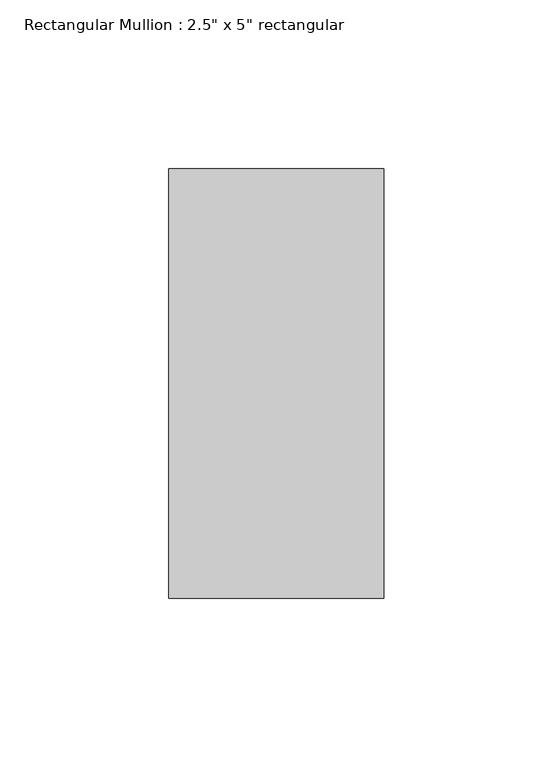
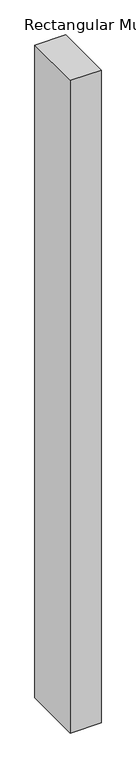
"""IFC4 building model written with IfcOpenShell, lengths in millimetres: member geometry."""

from ifc_helpers import new_model, si_unit, frame, origin, place, context, project, spatial, polyline, outline, extrude, source, transform, mapped, element, save


def member_26d67f61(model_context):
    return source(origin(), model_context, "Body", "SweptSolid", [
        extrude(outline(polyline([(0.0, 63.5), (0.0, -63.5), (-63.5, -63.5), (-63.5, 63.5), (0.0, 63.5)])), frame((0.0, 0.0, -1428.75), z_axis=(0.0, 0.0, 1.0), x_axis=(1.0, 0.0, 0.0)), (0.0, 0.0, 1.0), 1428.75),
    ])


if __name__ == "__main__":
    model = new_model("IFC4")
    model_context = context("Model", 3, world=origin())
    ifc_project = project(units=[si_unit("LENGTHUNIT", "METRE", prefix="MILLI")], contexts=[model_context])
    site = spatial("IfcSite", under=ifc_project)
    building = spatial("IfcBuilding", under=site)
    placement = place(None, origin())
    member_shape = member_26d67f61(model_context)
    element("IfcMember", 1, ObjectType="Rectangular Mullion : 2.5\" x 5\" rectangular", at=placement, inside=building, context=model_context, shape_type="MappedRepresentation", body=[
        mapped(member_shape, transform((0.0, 0.0, 0.0), x_axis=(1.0, 0.0, 0.0), y_axis=(0.0, 1.0, 0.0), z_axis=(0.0, 0.0, 1.0))),
    ])
    save(model, "model.ifc")

# Revit data of these elements
# Type "Rectangular Mullion : 2.5\" x 5\" rectangular"
#   built-in parameter 1007304 = 0.416667 (stored number, unit not read)
#   built-in parameter 1007301 = 0.104167 (stored number, unit not read)
#   built-in parameter 1007300 = 0.104167 (stored number, unit not read)
# Element 1 (IfcMember, "Rectangular Mullion : 2.5\" x 5\" rectangular")
#   Materials on its faces: "Rectangle 1 sq"
# Materials
#   "Rectangle 1 sq": class "Generic", colour RGB 120 120 120, transparency 0, Cost = 0
